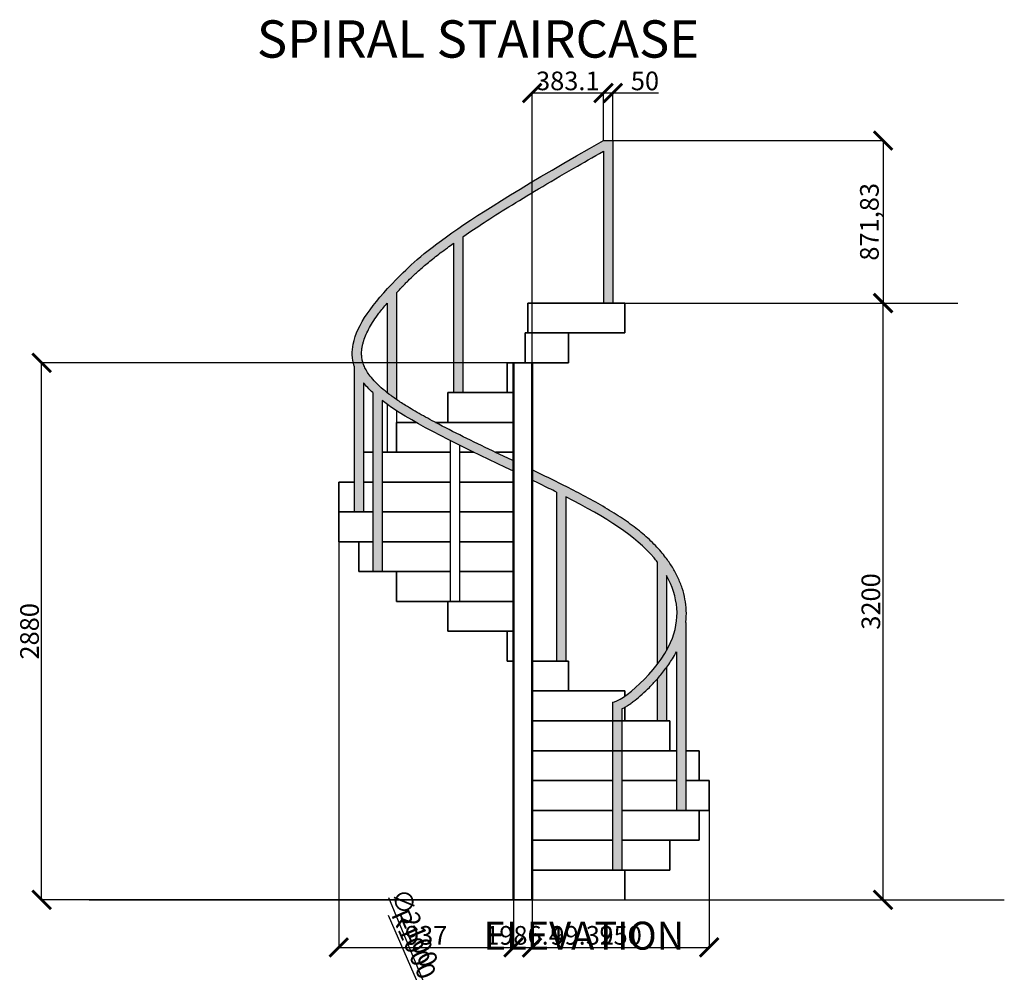
# Model space of a CAD drawing. Units: millimetres. Extents: x 210 to 5648, y 83 to 7906.
# Tile 2 of 2: x 210 to 5490, y 2798 to 7906. Entities that reach past the tile are written whole.
import ezdxf

# ---------------------------------------------------------------- set-up
doc = ezdxf.new("R2010")
doc.units = ezdxf.units.MM
for name, color, linetype, lineweight in [('A-ANNO-DIMS', 2, 'Continuous', 18), ('A-ANNO-TEXT', 240, 'Continuous', 18), ('A-COLS', 1, 'Continuous', 50), ('A-FLOR-HRAL', 4, 'Continuous', 25), ('A-FLOR-LEVL', 8, 'Continuous', 25), ('A-FLOR-PATT', 252, 'Continuous', 13), ('A-FLOR-STRS', 7, 'Continuous', 35)]:
    doc.layers.add(name, color=color, linetype=linetype, lineweight=lineweight)
doc.styles.get("Standard").update_dxf_attribs({"font": 'arial.ttf'})
doc.dimstyles.new('ISO-25', dxfattribs={"dimtxt": 100, "dimasz": 100, "dimexe": 1.25, "dimexo": 0.625, "dimtad": 1, "dimtxsty": 'Standard', "dimblk": 'ARCHTICK', "dimcen": 2.5, "dimclrd": 2, "dimclre": 5, "dimclrt": 1, "dimadec": 0, "dimazin": 0, "dimtfac": 1, "dimtmove": 0, "dimatfit": 3, "dimfxl": 1, "dimarcsym": 0})

# ---------------------------------------------------------------- blocks, each defined once
blk = doc.blocks.new('_ArchTick')
at = {"color": 0, "linetype": 'ByBlock', "const_width": 0.15}
blk.add_lwpolyline([(-0.5, -0.5), (0.5, 0.5)], dxfattribs=at)
blk = doc.blocks.new('*D4')
at = {"layer": 'A-ANNO-DIMS', "color": 0, "lineweight": -2, "transparency": 16777216}
for p, q in [((4348, 6386.1), (4839.8, 6386.1)), ((4838.6, 6386.1), (4838.6, 3186.1)), ((4348, 3186.1), (4839.8, 3186.1))]:
    blk.add_line(p, q, dxfattribs=at)
at = {"layer": 'Defpoints', "color": 0, "transparency": 16777216}
for p in [(4347.4, 6386.1), (4347.4, 3186.1), (4838.6, 3186.1)]:
    blk.add_point(p, dxfattribs=at)
at = {"layer": 'A-ANNO-DIMS', "color": 0, "lineweight": -2, "transparency": 16777216, "xscale": 100, "yscale": 100, "zscale": 100}
for p, rotation in [((4838.6, 6386.1), 90), ((4838.6, 3186.1), 270)]:
    blk.add_blockref('_ArchTick', p, dxfattribs=dict(at, rotation=rotation))
at = {"layer": 'A-ANNO-DIMS', "color": 0, "transparency": 16777216, "insert": (4786.9, 4786.1), "char_height": 100, "attachment_point": 5, "rotation": 90}
blk.add_mtext('3200', dxfattribs=at)
blk = doc.blocks.new('*D5')
at = {"layer": 'A-ANNO-DIMS', "color": 0, "lineweight": -2, "transparency": 16777216}
for p, q in [((3391.1, 7257.9), (4841.1, 7257.9)), ((4839.8, 7257.9), (4839.8, 6386.1)), ((3391.1, 6386.1), (4841.1, 6386.1))]:
    blk.add_line(p, q, dxfattribs=at)
at = {"layer": 'Defpoints', "color": 0, "transparency": 16777216}
for p in [(3390.5, 7257.9), (3390.5, 6386.1), (4839.8, 6386.1)]:
    blk.add_point(p, dxfattribs=at)
at = {"layer": 'A-ANNO-DIMS', "color": 0, "lineweight": -2, "transparency": 16777216, "xscale": 100, "yscale": 100, "zscale": 100}
for p, rotation in [((4839.8, 7257.9), 90), ((4839.8, 6386.1), 270)]:
    blk.add_blockref('_ArchTick', p, dxfattribs=dict(at, rotation=rotation))
at = {"layer": 'A-ANNO-DIMS', "color": 0, "transparency": 16777216, "insert": (4779.1, 6822), "char_height": 100, "attachment_point": 5, "rotation": 90}
blk.add_mtext('871,83', dxfattribs=at)
blk = doc.blocks.new('*D9')
at = {"layer": 'A-ANNO-DIMS', "color": 5, "lineweight": -2, "transparency": 16777216}
for p, q in [((2957.4, 6066.7), (2957.4, 7514.2)), ((3340.5, 7258.6), (3340.5, 7514.2))]:
    blk.add_line(p, q, dxfattribs=at)
at = {"layer": 'A-ANNO-DIMS', "color": 2, "lineweight": -2, "transparency": 16777216}
blk.add_line((2957.4, 7512.9), (3340.5, 7512.9), dxfattribs=at)
at = {"layer": 'Defpoints', "color": 0, "transparency": 16777216}
for p in [(3340.5, 7512.9), (3340.5, 7257.9), (2957.4, 6066.1)]:
    blk.add_point(p, dxfattribs=at)
at = {"layer": 'A-ANNO-DIMS', "color": 2, "lineweight": -2, "transparency": 16777216, "xscale": 100, "yscale": 100, "zscale": 100, "rotation": 180}
blk.add_blockref('_ArchTick', (2957.4, 7512.9), dxfattribs=at)
at = {"layer": 'A-ANNO-DIMS', "color": 2, "lineweight": -2, "transparency": 16777216, "xscale": 100, "yscale": 100, "zscale": 100}
blk.add_blockref('_ArchTick', (3340.5, 7512.9), dxfattribs=at)
at = {"layer": 'A-ANNO-DIMS', "color": 1, "transparency": 16777216, "insert": (3149, 7564.7), "char_height": 100, "attachment_point": 5}
blk.add_mtext('383.1', dxfattribs=at)
blk = doc.blocks.new('*D10')
at = {"layer": 'A-ANNO-DIMS', "color": 5, "lineweight": -2, "transparency": 16777216}
for p, q in [((3340.5, 7258.6), (3340.5, 7514.2)), ((3390.5, 7258.6), (3390.5, 7514.2))]:
    blk.add_line(p, q, dxfattribs=at)
at = {"layer": 'A-ANNO-DIMS', "color": 2, "lineweight": -2, "transparency": 16777216}
for p, q in [((3340.5, 7512.9), (3390.5, 7512.9)), ((3390.5, 7512.9), (3634.7, 7512.9))]:
    blk.add_line(p, q, dxfattribs=at)
at = {"layer": 'Defpoints', "color": 0, "transparency": 16777216}
for p in [(3390.5, 7512.9), (3340.5, 7257.9), (3390.5, 7257.9)]:
    blk.add_point(p, dxfattribs=at)
at = {"layer": 'A-ANNO-DIMS', "color": 2, "lineweight": -2, "transparency": 16777216, "xscale": 100, "yscale": 100, "zscale": 100, "rotation": 180}
blk.add_blockref('_ArchTick', (3340.5, 7512.9), dxfattribs=at)
at = {"layer": 'A-ANNO-DIMS', "color": 2, "lineweight": -2, "transparency": 16777216, "xscale": 100, "yscale": 100, "zscale": 100}
blk.add_blockref('_ArchTick', (3390.5, 7512.9), dxfattribs=at)
at = {"layer": 'A-ANNO-DIMS', "color": 1, "transparency": 16777216, "insert": (3562.6, 7564.6), "char_height": 100, "attachment_point": 5}
blk.add_mtext('50', dxfattribs=at)
blk = doc.blocks.new('*D11')
at = {"layer": 'A-ANNO-DIMS', "color": 5, "lineweight": -2, "transparency": 16777216}
for p, q in [((2957.4, 3825.5), (2957.4, 2929.9)), ((3907.4, 3825.5), (3907.4, 2929.9))]:
    blk.add_line(p, q, dxfattribs=at)
at = {"layer": 'A-ANNO-DIMS', "color": 2, "lineweight": -2, "transparency": 16777216}
blk.add_line((2957.4, 2931.1), (3907.4, 2931.1), dxfattribs=at)
at = {"layer": 'Defpoints', "color": 0, "transparency": 16777216}
for p in [(2957.4, 3826.1), (3907.4, 3826.1), (3907.4, 2931.1)]:
    blk.add_point(p, dxfattribs=at)
at = {"layer": 'A-ANNO-DIMS', "color": 2, "lineweight": -2, "transparency": 16777216, "xscale": 100, "yscale": 100, "zscale": 100, "rotation": 180}
blk.add_blockref('_ArchTick', (2957.4, 2931.1), dxfattribs=at)
at = {"layer": 'A-ANNO-DIMS', "color": 2, "lineweight": -2, "transparency": 16777216, "xscale": 100, "yscale": 100, "zscale": 100}
blk.add_blockref('_ArchTick', (3907.4, 2931.1), dxfattribs=at)
at = {"layer": 'A-ANNO-DIMS', "color": 1, "transparency": 16777216, "insert": (3432.4, 2982.8), "char_height": 100, "attachment_point": 5}
blk.add_mtext('950', dxfattribs=at)
blk = doc.blocks.new('*D12')
at = {"layer": 'A-ANNO-DIMS', "color": 5, "lineweight": -2, "transparency": 16777216}
for p, q in [((1921, 5105.5), (1921, 2929.9)), ((2858.1, 5105.5), (2858.1, 2929.9))]:
    blk.add_line(p, q, dxfattribs=at)
at = {"layer": 'A-ANNO-DIMS', "color": 2, "lineweight": -2, "transparency": 16777216}
blk.add_line((1921, 2931.1), (2858.1, 2931.1), dxfattribs=at)
at = {"layer": 'Defpoints', "color": 0, "transparency": 16777216}
for p in [(1921, 5106.1), (2858.1, 5106.1), (2858.1, 2931.1)]:
    blk.add_point(p, dxfattribs=at)
at = {"layer": 'A-ANNO-DIMS', "color": 2, "lineweight": -2, "transparency": 16777216, "xscale": 100, "yscale": 100, "zscale": 100, "rotation": 180}
blk.add_blockref('_ArchTick', (1921, 2931.1), dxfattribs=at)
at = {"layer": 'A-ANNO-DIMS', "color": 2, "lineweight": -2, "transparency": 16777216, "xscale": 100, "yscale": 100, "zscale": 100}
blk.add_blockref('_ArchTick', (2858.1, 2931.1), dxfattribs=at)
at = {"layer": 'A-ANNO-DIMS', "color": 1, "transparency": 16777216, "insert": (2389.6, 2982.8), "char_height": 100, "attachment_point": 5}
blk.add_mtext('937', dxfattribs=at)
blk = doc.blocks.new('*D13')
at = {"layer": 'A-ANNO-DIMS', "color": 5, "lineweight": -2, "transparency": 16777216}
for p, q in [((2858.1, 3185.5), (2858.1, 2929.9)), ((2957.4, 3185.5), (2957.4, 2929.9))]:
    blk.add_line(p, q, dxfattribs=at)
at = {"layer": 'A-ANNO-DIMS', "color": 2, "lineweight": -2, "transparency": 16777216}
for p, q in [((2858.1, 2931.1), (2957.4, 2931.1)), ((2957.4, 2931.1), (3395.1, 2931.1))]:
    blk.add_line(p, q, dxfattribs=at)
at = {"layer": 'Defpoints', "color": 0, "transparency": 16777216}
for p in [(2858.1, 3186.1), (2957.4, 3186.1), (2957.4, 2931.1)]:
    blk.add_point(p, dxfattribs=at)
at = {"layer": 'A-ANNO-DIMS', "color": 2, "lineweight": -2, "transparency": 16777216, "xscale": 100, "yscale": 100, "zscale": 100, "rotation": 180}
blk.add_blockref('_ArchTick', (2858.1, 2931.1), dxfattribs=at)
at = {"layer": 'A-ANNO-DIMS', "color": 2, "lineweight": -2, "transparency": 16777216, "xscale": 100, "yscale": 100, "zscale": 100}
blk.add_blockref('_ArchTick', (2957.4, 2931.1), dxfattribs=at)
at = {"layer": 'A-ANNO-DIMS', "color": 1, "transparency": 16777216, "insert": (3226.2, 2982.8), "char_height": 100, "attachment_point": 5}
blk.add_mtext('99.32', dxfattribs=at)
blk = doc.blocks.new('*D14')
at = {"layer": 'A-ANNO-DIMS', "color": 5, "lineweight": -2, "transparency": 16777216}
for p, q in [((1921, 5265.5), (1921, 2929.9)), ((3907.4, 3665.5), (3907.4, 2929.9))]:
    blk.add_line(p, q, dxfattribs=at)
at = {"layer": 'A-ANNO-DIMS', "color": 2, "lineweight": -2, "transparency": 16777216}
blk.add_line((1921, 2931.1), (3907.4, 2931.1), dxfattribs=at)
at = {"layer": 'Defpoints', "color": 0, "transparency": 16777216}
for p in [(1921, 5266.1), (3907.4, 3666.1), (3907.4, 2931.1)]:
    blk.add_point(p, dxfattribs=at)
at = {"layer": 'A-ANNO-DIMS', "color": 2, "lineweight": -2, "transparency": 16777216, "xscale": 100, "yscale": 100, "zscale": 100, "rotation": 180}
blk.add_blockref('_ArchTick', (1921, 2931.1), dxfattribs=at)
at = {"layer": 'A-ANNO-DIMS', "color": 2, "lineweight": -2, "transparency": 16777216, "xscale": 100, "yscale": 100, "zscale": 100}
blk.add_blockref('_ArchTick', (3907.4, 2931.1), dxfattribs=at)
at = {"layer": 'A-ANNO-DIMS', "color": 1, "transparency": 16777216, "insert": (2914.2, 2982.8), "char_height": 100, "attachment_point": 5}
blk.add_mtext('1986.4', dxfattribs=at)
blk = doc.blocks.new('*D15')
at = {"layer": 'A-ANNO-DIMS', "color": 5, "lineweight": -2, "transparency": 16777216}
for p, q in [((2956.8, 6066.1), (326.4, 6066.1)), ((2956.8, 3186.1), (326.4, 3186.1))]:
    blk.add_line(p, q, dxfattribs=at)
at = {"layer": 'A-ANNO-DIMS', "color": 2, "lineweight": -2, "transparency": 16777216}
blk.add_line((327.6, 3186.1), (327.6, 6066.1), dxfattribs=at)
at = {"layer": 'Defpoints', "color": 0, "transparency": 16777216}
for p in [(327.6, 6066.1), (2957.4, 6066.1), (2957.4, 3186.1)]:
    blk.add_point(p, dxfattribs=at)
at = {"layer": 'A-ANNO-DIMS', "color": 2, "lineweight": -2, "transparency": 16777216, "xscale": 100, "yscale": 100, "zscale": 100}
for p, rotation in [((327.6, 6066.1), 90), ((327.6, 3186.1), 270)]:
    blk.add_blockref('_ArchTick', p, dxfattribs=dict(at, rotation=rotation))
at = {"layer": 'A-ANNO-DIMS', "color": 1, "transparency": 16777216, "insert": (275.9, 4626.1), "char_height": 100, "attachment_point": 5, "rotation": 90}
blk.add_mtext('2880', dxfattribs=at)
blk = doc.blocks.new('*D16')
at = {"layer": 'A-ANNO-DIMS', "color": 2, "lineweight": -2, "transparency": 16777216}
for p in [(2187.7, 3199), (3308.5, 487.3)]:
    blk.add_line(p, (2506.3, 2428.1), dxfattribs=at)
at = {"layer": 'Defpoints', "color": 0, "transparency": 16777216}
for p in [(2506.3, 2428.1), (3308.5, 487.3)]:
    blk.add_point(p, dxfattribs=at)
at = {"layer": 'A-ANNO-DIMS', "color": 2, "lineweight": -2, "transparency": 16777216, "xscale": 100, "yscale": 100, "zscale": 100}
for p, rotation in [((2506.3, 2428.1), 292.4567190753457), ((3308.5, 487.3), 112.4567190753456)]:
    blk.add_blockref('_ArchTick', p, dxfattribs=dict(at, rotation=rotation))
at = {"layer": 'A-ANNO-DIMS', "color": 1, "transparency": 16777216, "insert": (2316, 3031.1), "char_height": 100, "attachment_point": 5, "rotation": 292.4567}
blk.add_mtext('∅2100', dxfattribs=at)
blk = doc.blocks.new('*D17')
at = {"layer": 'A-ANNO-DIMS', "color": 2, "lineweight": -2, "transparency": 16777216}
for p in [(2185.3, 3103.9), (2907.4, 1457.7)]:
    blk.add_line(p, (2505.7, 2373.5), dxfattribs=at)
at = {"layer": 'Defpoints', "color": 0, "transparency": 16777216}
for p in [(2505.7, 2373.5), (2907.4, 1457.7)]:
    blk.add_point(p, dxfattribs=at)
at = {"layer": 'A-ANNO-DIMS', "color": 2, "lineweight": -2, "transparency": 16777216, "xscale": 100, "yscale": 100, "zscale": 100, "rotation": 293.6842151788714}
blk.add_blockref('_ArchTick', (2505.7, 2373.5), dxfattribs=at)
at = {"layer": 'A-ANNO-DIMS', "color": 1, "transparency": 16777216, "insert": (2312, 2943.7), "char_height": 100, "attachment_point": 5, "rotation": 293.6842}
blk.add_mtext('R1000', dxfattribs=at)

msp = doc.modelspace()

# ---------------------------------------------------------------- hatches: boundary and pattern name
at = {"layer": 'A-FLOR-PATT'}
h = msp.add_hatch(color=256, dxfattribs=at)
h.dxf.hatch_style = 1
edge = h.paths.add_edge_path()
edge.add_spline(control_points=[(2230.323, 6441.345), (2237.214, 6448.743), (2244.288, 6456.237), (2254.94, 6467.39), (2258.378, 6470.97), (2264.36, 6477.168), (2266.887, 6479.777), (2271.968, 6485.002), (2274.525, 6487.621), (2282.261, 6495.505), (2287.506, 6500.797), (2303.631, 6516.855), (2314.902, 6527.799), (2341.337, 6552.563), (2356.838, 6566.548), (2391.369, 6596.276), (2410.399, 6612.017), (2453.073, 6645.774), (2476.716, 6663.789), (2513.779, 6690.939), (2524.82, 6698.916), (2536.348, 6707.128)], knot_values=[5.90489117, 5.90489117, 5.90489117, 5.90489117, 5.96373465, 5.96373465, 5.9913029, 5.9913029, 6.0111685, 6.0111685, 6.03103409, 6.03103409, 6.07076529, 6.07076529, 6.15022769, 6.15022769, 6.24382005, 6.24382005, 6.33741241, 6.33741241, 6.43100477, 6.43100477, 6.46843693, 6.46843693, 6.46843693, 6.46843693], degree=3, periodic=0)
edge.add_line((2536.348, 6707.128), (2536.348, 5906.102))
edge.add_line((2536.348, 5906.102), (2586.348, 5906.102))
edge.add_line((2586.348, 5906.102), (2586.348, 6742.111))
edge.add_spline(control_points=[(2586.348, 6742.111), (2588.096, 6743.314), (2589.855, 6744.521), (2657.298, 6790.759), (2736.51, 6842.312), (2930.306, 6962.284), (3044.888, 7030.703), (3231.366, 7138.39), (3284.371, 7168.696), (3340.522, 7200.493)], knot_values=[6.51952859, 6.51952859, 6.51952859, 6.51952859, 6.52459713, 6.52459713, 6.71284254, 6.71284254, 6.90108795, 6.90108795, 6.97017576, 6.97017576, 6.97017576, 6.97017576], degree=3, periodic=0)
edge.add_line((3340.522, 7200.493), (3340.522, 6386.102))
edge.add_line((3340.522, 6386.102), (3390.522, 6386.102))
edge.add_line((3390.522, 6386.102), (3390.522, 7257.935))
edge.add_line((3390.522, 7257.935), (3340.522, 7257.935))
edge.add_spline(control_points=[(3340.522, 7257.935), (2981.042, 7054.904), (2746.784, 6911.149), (2586.348, 6802.632)], knot_values=[6.54582273, 6.54582273, 6.54582273, 6.54582273, 6.98017889, 6.98017889, 6.98017889, 6.98017889], degree=3, periodic=0)
edge.add_spline(control_points=[(2586.348, 6802.632), (2384.739, 6666.266), (2143.904, 6437.657), (1990.881, 6234.097), (1991.101, 6088.759), (2003.82, 6048.816)], knot_values=[4.63745133, 4.63745133, 4.63745133, 4.63745133, 5.18327406, 6.18327406, 6.54582273, 6.54582273, 6.54582273, 6.54582273], degree=3, periodic=0)
edge.add_line((2003.82, 6048.816), (2003.82, 5266.102))
edge.add_line((2003.82, 5266.102), (2053.82, 5266.102))
edge.add_line((2053.82, 5266.102), (2053.82, 5958.825))
edge.add_spline(control_points=[(2053.82, 5958.825), (2067.467, 5941.686), (2083.758, 5924.189), (2103.017, 5906.251)], knot_values=[4.2265259, 4.2265259, 4.2265259, 4.2265259, 4.37281832, 4.37281832, 4.37281832, 4.37281832], degree=3, periodic=0)
edge.add_line((2103.017, 5906.251), (2103.017, 4946.102))
edge.add_line((2103.017, 4946.102), (2153.017, 4946.102))
edge.add_line((2153.017, 4946.102), (2153.017, 5863.924))
edge.add_spline(control_points=[(2153.017, 5863.924), (2161.695, 5857.182), (2170.791, 5850.374), (2180.323, 5843.497)], knot_values=[4.06087851, 4.06087851, 4.06087851, 4.06087851, 4.11370793, 4.11370793, 4.11370793, 4.11370793], degree=3, periodic=0)
edge.add_spline(control_points=[(2180.323, 5843.497), (2191.306, 5835.571), (2207.618, 5824.257), (2225.126, 5812.747), (2230.323, 5809.378)], knot_values=[3.97497946, 3.97497946, 3.97497946, 3.97497946, 4.03585797, 4.06087851, 4.06087851, 4.06087851, 4.06087851], degree=3, periodic=0)
edge.add_spline(control_points=[(2230.323, 5809.378), (2262.049, 5788.814), (2297.407, 5767.659), (2335.496, 5746.102)], knot_values=[3.8222376, 3.8222376, 3.8222376, 3.8222376, 3.97497946, 3.97497946, 3.97497946, 3.97497946], degree=3, periodic=0)
edge.add_spline(control_points=[(2335.496, 5746.102), (2391.715, 5714.285), (2453.883, 5681.595), (2519.103, 5648.642)], knot_values=[3.59679122, 3.59679122, 3.59679122, 3.59679122, 3.8222376, 3.8222376, 3.8222376, 3.8222376], degree=3, periodic=0)
edge.add_spline(control_points=[(2519.103, 5648.642), (2535.59, 5640.312), (2552.272, 5631.965), (2569.103, 5623.611)], knot_values=[3.53979942, 3.53979942, 3.53979942, 3.53979942, 3.59679122, 3.59679122, 3.59679122, 3.59679122], degree=3, periodic=0)
edge.add_spline(control_points=[(2569.103, 5623.611), (2594.283, 5611.112), (2619.795, 5598.598), (2645.481, 5586.102)], knot_values=[3.45453406, 3.45453406, 3.45453406, 3.45453406, 3.53979942, 3.53979942, 3.53979942, 3.53979942], degree=3, periodic=0)
edge.add_spline(control_points=[(2645.481, 5586.102), (2716.113, 5551.741), (2788.067, 5517.513), (2858.085, 5484.105)], knot_values=[3.22007561, 3.22007561, 3.22007561, 3.22007561, 3.45453406, 3.45453406, 3.45453406, 3.45453406], degree=3, periodic=0)
edge.add_line((2858.085, 5484.105), (2858.085, 5539.503))
edge.add_spline(control_points=[(2858.085, 5539.503), (2827.328, 5554.173), (2796.294, 5568.971), (2763.683, 5584.596), (2762.111, 5585.349), (2760.54, 5586.102)], knot_values=[3.24403738, 3.24403738, 3.24403738, 3.24403738, 3.34649082, 3.34649082, 3.35167775, 3.35167775, 3.35167775, 3.35167775], degree=3, periodic=0)
edge.add_spline(control_points=[(2760.54, 5586.102), (2709.179, 5610.722), (2657.838, 5635.532), (2556.156, 5685.75), (2505.893, 5711.154), (2452.051, 5739.479), (2445.783, 5742.795), (2439.567, 5746.102)], knot_values=[3.35167775, 3.35167775, 3.35167775, 3.35167775, 3.52120514, 3.52120514, 3.69591945, 3.69591945, 3.71913913, 3.71913913, 3.71913913, 3.71913913], degree=3, periodic=0)
edge.add_spline(control_points=[(2439.567, 5746.102), (2413.223, 5760.121), (2387.808, 5773.996), (2333.635, 5804.555), (2305.503, 5821.132), (2269.838, 5843.389), (2260.321, 5849.471), (2243.996, 5860.182), (2237.049, 5864.841), (2230.323, 5869.455)], knot_values=[3.71913913, 3.71913913, 3.71913913, 3.71913913, 3.81754541, 3.81754541, 3.93917136, 3.93917136, 3.98562211, 3.98562211, 4.02206941, 4.02206941, 4.02206941, 4.02206941], degree=3, periodic=0)
edge.add_spline(control_points=[(2230.323, 5869.455), (2228.581, 5870.65), (2226.854, 5871.842), (2216.818, 5878.81), (2208.841, 5884.519), (2193.939, 5895.516), (2186.982, 5900.811), (2180.323, 5906.041)], knot_values=[4.02206941, 4.02206941, 4.02206941, 4.02206941, 4.03150589, 4.03150589, 4.07738967, 4.07738967, 4.12101551, 4.12101551, 4.12101551, 4.12101551], degree=3, periodic=0)
edge.add_spline(control_points=[(2180.323, 5906.041), (2172.974, 5911.812), (2165.987, 5917.504), (2144.201, 5935.928), (2130.878, 5948.324), (2107.575, 5972.254), (2097.596, 5983.788), (2082.165, 6003.935), (2076.218, 6012.694), (2066.046, 6029.662), (2061.82, 6037.87), (2054.825, 6053.836), (2052.053, 6061.594), (2047.722, 6076.837), (2046.161, 6084.324), (2044.077, 6099.249), (2043.555, 6106.689), (2043.453, 6121.725), (2043.876, 6129.321), (2045.161, 6140.725), (2045.674, 6144.419), (2046.77, 6151.11), (2047.318, 6154.096), (2048.532, 6160.108), (2049.197, 6163.123), (2051.367, 6172.201), (2053.047, 6178.299), (2058.458, 6195.653), (2062.743, 6207.05), (2072.966, 6230.362), (2078.906, 6242.275), (2092.479, 6266.689), (2100.113, 6279.188), (2117.083, 6304.82), (2126.418, 6317.953), (2149.772, 6348.873), (2164.362, 6366.889), (2180.323, 6385.536)], knot_values=[4.12101551, 4.12101551, 4.12101551, 4.12101551, 4.16915722, 4.16915722, 4.27905295, 4.27905295, 4.38894868, 4.38894868, 4.4785858, 4.4785858, 4.56822292, 4.56822292, 4.65786004, 4.65786004, 4.74749715, 4.74749715, 4.83713427, 4.83713427, 4.92677139, 4.92677139, 4.96916501, 4.96916501, 5.00281636, 5.00281636, 5.03646771, 5.03646771, 5.1037704, 5.1037704, 5.22617685, 5.22617685, 5.34858331, 5.34858331, 5.47098976, 5.47098976, 5.59339622, 5.59339622, 5.75191312, 5.75191312, 5.75191312, 5.75191312], degree=3, periodic=0)
edge.add_line((2180.323, 6385.536), (2180.323, 5906.041))
edge.add_spline(control_points=[(2180.323, 5906.041), (2186.982, 5900.811), (2193.939, 5895.516), (2208.841, 5884.519), (2216.818, 5878.81), (2226.854, 5871.842), (2228.581, 5870.65), (2230.323, 5869.455)], knot_values=[4.02206941, 4.02206941, 4.02206941, 4.02206941, 4.06569525, 4.06569525, 4.11157903, 4.11157903, 4.12101551, 4.12101551, 4.12101551, 4.12101551], degree=3, periodic=0)
edge.add_line((2230.323, 5869.455), (2230.323, 6441.345))
h = msp.add_hatch(color=256, dxfattribs=at)
h.dxf.hatch_style = 1
edge = h.paths.add_edge_path()
edge.add_spline(control_points=[(3781.861, 4673.689), (3781.945, 4674.405), (3782.026, 4675.121), (3784.412, 4696.601), (3785.116, 4717.29), (3783.499, 4758.294), (3781.181, 4778.609), (3773.753, 4818.679), (3768.645, 4838.436), (3755.889, 4877.258), (3748.241, 4896.325), (3730.647, 4933.684), (3720.701, 4951.976), (3698.73, 4987.728), (3686.706, 5005.188), (3665.888, 5032.519), (3657.69, 5042.669), (3629.972, 5075.136), (3609.122, 5096.786), (3564.067, 5138.823), (3539.863, 5159.212), (3487.997, 5199.2), (3460.335, 5218.801), (3401.383, 5257.702), (3370.093, 5277.003), (3303.681, 5315.786), (3268.56, 5335.267), (3214.918, 5363.864), (3198.024, 5372.72), (3146.116, 5399.538), (3109.873, 5417.749), (3035.144, 5454.562), (2996.77, 5473.13), (2957.403, 5492.028)], knot_values=[1.23691972, 1.23691972, 1.23691972, 1.23691972, 1.24089242, 1.24089242, 1.35609231, 1.35609231, 1.4712922, 1.4712922, 1.58649209, 1.58649209, 1.70169198, 1.70169198, 1.81689187, 1.81689187, 1.93209176, 1.93209176, 2.00188444, 2.00188444, 2.15904986, 2.15904986, 2.31621528, 2.31621528, 2.47338069, 2.47338069, 2.63054611, 2.63054611, 2.78771153, 2.78771153, 2.85749508, 2.85749508, 2.99706219, 2.99706219, 3.13226931, 3.13226931, 3.13226931, 3.13226931], degree=3, periodic=0)
edge.add_line((2957.403, 5492.028), (2957.403, 5436.549))
edge.add_spline(control_points=[(2957.403, 5436.549), (2988.252, 5421.693), (3032.736, 5400.104), (3074.935, 5379.185), (3088.331, 5372.491)], knot_values=[2.94879845, 2.94879845, 2.94879845, 2.94879845, 3.05611076, 3.10731232, 3.10731232, 3.10731232, 3.10731232], degree=3, periodic=0)
edge.add_line((3088.331, 5372.491), (3088.331, 4466.102))
edge.add_line((3088.331, 4466.102), (3138.331, 4466.102))
edge.add_line((3138.331, 4466.102), (3138.331, 5347.228))
edge.add_spline(control_points=[(3138.331, 5347.228), (3359.291, 5234.253), (3520.089, 5131.778), (3622.943, 5006.062), (3628.268, 4999.279)], knot_values=[1.95009854, 1.95009854, 1.95009854, 1.95009854, 2.83374836, 2.88364982, 2.88364982, 2.88364982, 2.88364982], degree=3, periodic=0)
edge.add_line((3628.268, 4999.279), (3628.268, 4448.446))
edge.add_spline(control_points=[(3628.268, 4448.446), (3646.667, 4472.431), (3663.687, 4497.441), (3678.268, 4522.82)], knot_values=[0.74965342, 0.74965342, 0.74965342, 0.74965342, 0.90958311, 0.90958311, 0.90958311, 0.90958311], degree=3, periodic=0)
edge.add_line((3678.268, 4522.82), (3678.268, 4924.666))
edge.add_spline(control_points=[(3678.268, 4924.666), (3740.506, 4813.344), (3757.759, 4675.257), (3686.512, 4537.169), (3678.268, 4522.82)], knot_values=[0.90958311, 0.90958311, 0.90958311, 0.90958311, 1.68221449, 1.77263138, 1.77263138, 1.77263138, 1.77263138], degree=3, periodic=0)
edge.add_spline(control_points=[(3678.268, 4522.82), (3663.687, 4497.441), (3646.667, 4472.431), (3628.268, 4448.446)], knot_values=[0.74965342, 0.74965342, 0.74965342, 0.74965342, 0.90958311, 0.90958311, 0.90958311, 0.90958311], degree=3, periodic=0)
edge.add_spline(control_points=[(3628.268, 4448.446), (3573.149, 4376.59), (3505.665, 4313.928), (3454.351, 4278.062)], knot_values=[0.27051991, 0.27051991, 0.27051991, 0.27051991, 0.74965342, 0.74965342, 0.74965342, 0.74965342], degree=3, periodic=0)
edge.add_spline(control_points=[(3454.351, 4278.062), (3425.379, 4257.811), (3401.562, 4246.102), (3388.036, 4246.102)], knot_values=[0, 0, 0, 0, 0.27051991, 0.27051991, 0.27051991, 0.27051991], degree=3, periodic=0)
edge.add_line((3388.036, 4245.424), (3388.036, 4146.102))
edge.add_line((3388.036, 4146.102), (3438.036, 4146.102))
edge.add_line((3438.036, 4146.102), (3438.036, 4209.897))
edge.add_spline(control_points=[(3438.036, 4209.897), (3440.677, 4211.191), (3443.321, 4212.552), (3448.752, 4215.468), (3451.54, 4217.029), (3454.351, 4218.661)], knot_values=[0.13781612, 0.13781612, 0.13781612, 0.13781612, 0.1620919, 0.1620919, 0.18736587, 0.18736587, 0.18736587, 0.18736587], degree=3, periodic=0)
edge.add_spline(control_points=[(3454.351, 4218.661), (3454.757, 4218.897), (3455.163, 4219.134), (3461.214, 4222.683), (3466.96, 4226.282), (3478.698, 4234.043), (3484.688, 4238.205), (3496.903, 4247.07), (3503.128, 4251.773), (3521.788, 4266.405), (3534.509, 4277.057), (3560.369, 4300.091), (3573.506, 4312.474), (3599.764, 4338.724), (3612.886, 4352.59), (3626.606, 4368.011), (3627.438, 4368.949), (3628.268, 4369.891)], knot_values=[0.18736587, 0.18736587, 0.18736587, 0.18736587, 0.19101455, 0.19101455, 0.24163062, 0.24163062, 0.29224669, 0.29224669, 0.34286276, 0.34286276, 0.44154301, 0.44154301, 0.54022326, 0.54022326, 0.63890352, 0.63890352, 0.64528101, 0.64528101, 0.64528101, 0.64528101], degree=3, periodic=0)
edge.add_spline(control_points=[(3628.268, 4369.891), (3642.58, 4386.105), (3656.582, 4403.075), (3672.751, 4424.326), (3675.525, 4428.035), (3678.268, 4431.769)], knot_values=[0.64528101, 0.64528101, 0.64528101, 0.64528101, 0.75514118, 0.75514118, 0.77817085, 0.77817085, 0.77817085, 0.77817085], degree=3, periodic=0)
edge.add_spline(control_points=[(3678.268, 4431.769), (3689.371, 4446.881), (3699.966, 4462.403), (3717.67, 4490.805), (3725.045, 4503.562), (3731.861, 4516.498)], knot_values=[0.77817085, 0.77817085, 0.77817085, 0.77817085, 0.87137885, 0.87137885, 0.9451649, 0.9451649, 0.9451649, 0.9451649], degree=3, periodic=0)
edge.add_line((3731.861, 4516.498), (3731.861, 3666.102))
edge.add_line((3731.861, 3666.102), (3781.861, 3666.102))
edge.add_line((3781.861, 3666.102), (3781.861, 4673.689))
h.paths.add_polyline_path([(3438.036, 3986.102), (3388.036, 3986.102), (3388.036, 3346.102), (3438.036, 3346.102)])
h = msp.add_hatch(color=256, dxfattribs=at)
h.dxf.hatch_style = 1
edge = h.paths.add_edge_path()
edge.add_spline(control_points=[(3678.268, 4431.769), (3675.525, 4428.035), (3672.751, 4424.326), (3656.582, 4403.075), (3642.58, 4386.105), (3628.268, 4369.891)], knot_values=[0.64528101, 0.64528101, 0.64528101, 0.64528101, 0.66831067, 0.66831067, 0.77817085, 0.77817085, 0.77817085, 0.77817085], degree=3, periodic=0)
edge.add_line((3628.268, 4369.891), (3628.268, 4146.102))
edge.add_line((3628.268, 4146.102), (3678.268, 4146.102))
edge.add_line((3678.268, 4146.102), (3678.268, 4431.769))
h = msp.add_hatch(color=256, dxfattribs=at)
h.dxf.hatch_style = 1
h.paths.add_polyline_path([(3438.036, 4146.102), (3388.036, 4146.102), (3388.036, 3986.102), (3438.036, 3986.102)])

# ---------------------------------------------------------------- linework, layer by layer
at = {"layer": 'A-COLS'}
for p, q in [((2858.085, 5484.105), (2858.085, 6066.102)), ((2957.403, 5436.549), (2957.403, 6066.102)), ((2858.085, 3186.102), (2858.085, 5484.105)), ((2957.403, 3186.102), (2957.403, 5436.549))]:
    msp.add_line(p, q, dxfattribs=at)
at = {"layer": 'A-FLOR-HRAL'}
for p, q in [((3340.522, 7257.935), (3390.522, 7257.935)), ((3390.522, 7257.935), (3390.522, 6386.102)), ((3340.522, 7200.493), (3340.522, 6386.102)), ((2586.348, 6806.102), (2586.348, 6802.632)), ((2536.348, 6707.128), (2536.348, 5906.102)), ((2586.348, 6742.111), (2586.348, 5906.102)), ((2230.323, 6441.345), (2230.323, 5869.455)), ((2180.323, 6385.536), (2180.323, 5906.041)), ((2003.82, 6048.816), (2003.82, 5266.102)), ((2053.82, 5958.825), (2053.82, 5266.102)), ((2103.017, 5906.251), (2103.017, 4946.102)), ((2153.017, 5863.924), (2153.017, 4946.102)), ((2180.323, 5843.497), (2180.323, 5586.102)), ((2230.323, 5809.378), (2230.323, 5586.102)), ((2519.103, 5648.642), (2519.103, 4786.102)), ((2569.103, 5623.611), (2569.103, 4786.102)), ((3088.331, 5372.491), (3088.331, 4466.102)), ((3138.331, 5347.228), (3138.331, 4466.102)), ((3628.268, 4999.279), (3628.268, 4448.446)), ((3678.268, 4924.666), (3678.268, 4522.82)), ((3781.861, 4673.689), (3781.861, 3666.102)), ((3731.861, 4516.498), (3731.861, 3666.102)), ((3678.268, 4431.769), (3678.268, 4146.102)), ((3628.268, 4369.891), (3628.268, 4146.102)), ((3388.036, 4246.102), (3388.036, 3346.102)), ((3438.036, 4209.897), (3438.036, 3346.102))]:
    msp.add_line(p, q, dxfattribs=at)
for points, knots in [([(2003.82, 6048.816), (1991.101, 6088.759), (1990.881, 6234.097), (2178.733, 6483.988), (2529.31, 6799.77), (3340.522, 7257.935)], [4.63745133, 4.63745133, 4.63745133, 4.63745133, 5, 6, 6.98017889, 6.98017889, 6.98017889, 6.98017889]), ([(2586.348, 6742.111), (2588.096, 6743.314), (2589.855, 6744.521), (2657.298, 6790.759), (2736.51, 6842.312), (2930.306, 6962.284), (3044.888, 7030.703), (3231.366, 7138.39), (3284.371, 7168.696), (3340.522, 7200.493)], [6.519528589, 6.519528589, 6.519528589, 6.519528589, 6.524597131, 6.524597131, 6.712842542, 6.712842542, 6.901087953, 6.901087953, 6.970175759, 6.970175759, 6.970175759, 6.970175759]), ([(2230.323, 6441.345), (2237.214, 6448.743), (2244.288, 6456.237), (2254.94, 6467.39), (2258.378, 6470.97), (2264.36, 6477.168), (2266.887, 6479.777), (2271.968, 6485.002), (2274.525, 6487.621), (2282.261, 6495.505), (2287.506, 6500.797), (2303.631, 6516.855), (2314.902, 6527.799), (2341.337, 6552.563), (2356.838, 6566.548), (2391.369, 6596.276), (2410.399, 6612.017), (2453.073, 6645.774), (2476.716, 6663.789), (2513.779, 6690.939), (2524.82, 6698.916), (2536.348, 6707.128)], [5.904891169, 5.904891169, 5.904891169, 5.904891169, 5.963734651, 5.963734651, 5.991302897, 5.991302897, 6.011168496, 6.011168496, 6.031034094, 6.031034094, 6.070765292, 6.070765292, 6.150227687, 6.150227687, 6.243820048, 6.243820048, 6.337412409, 6.337412409, 6.43100477, 6.43100477, 6.468436926, 6.468436926, 6.468436926, 6.468436926]), ([(2858.085, 5539.503), (2827.328, 5554.173), (2796.294, 5568.971), (2712.321, 5609.204), (2659.37, 5634.775), (2556.156, 5685.75), (2505.893, 5711.154), (2425.282, 5753.561), (2393.525, 5770.771), (2333.635, 5804.555), (2305.503, 5821.132), (2269.838, 5843.389), (2260.321, 5849.471), (2242.137, 5861.402), (2233.467, 5867.25), (2216.818, 5878.81), (2208.841, 5884.519), (2185.925, 5901.43), (2172.001, 5912.418), (2144.201, 5935.928), (2130.878, 5948.324), (2107.575, 5972.254), (2097.596, 5983.788), (2082.165, 6003.935), (2076.218, 6012.694), (2066.046, 6029.662), (2061.82, 6037.87), (2054.825, 6053.836), (2052.053, 6061.594), (2047.722, 6076.837), (2046.161, 6084.324), (2044.077, 6099.249), (2043.555, 6106.689), (2043.453, 6121.725), (2043.876, 6129.321), (2045.161, 6140.725), (2045.674, 6144.419), (2046.77, 6151.11), (2047.318, 6154.096), (2048.532, 6160.108), (2049.197, 6163.123), (2051.367, 6172.201), (2053.047, 6178.299), (2058.458, 6195.653), (2062.743, 6207.05), (2072.966, 6230.362), (2078.906, 6242.275), (2092.479, 6266.689), (2100.113, 6279.188), (2117.083, 6304.82), (2126.418, 6317.953), (2149.772, 6348.873), (2164.362, 6366.889), (2180.323, 6385.536)], [3.24403738, 3.24403738, 3.24403738, 3.24403738, 3.34649082, 3.34649082, 3.52120514, 3.52120514, 3.69591945, 3.69591945, 3.81754541, 3.81754541, 3.93917136, 3.93917136, 3.98562211, 3.98562211, 4.03150589, 4.03150589, 4.07738967, 4.07738967, 4.16915722, 4.16915722, 4.27905295, 4.27905295, 4.38894868, 4.38894868, 4.4785858, 4.4785858, 4.56822292, 4.56822292, 4.65786004, 4.65786004, 4.74749715, 4.74749715, 4.83713427, 4.83713427, 4.92677139, 4.92677139, 4.96916501, 4.96916501, 5.00281636, 5.00281636, 5.03646771, 5.03646771, 5.1037704, 5.1037704, 5.22617685, 5.22617685, 5.34858331, 5.34858331, 5.47098976, 5.47098976, 5.59339622, 5.59339622, 5.75191312, 5.75191312, 5.75191312, 5.75191312]), ([(2858.085, 5484.105), (2625.173, 5595.235), (2333.744, 5732.972), (2171.694, 5849.413), (2153.017, 5863.924)], [3.220075614, 3.220075614, 3.220075614, 3.220075614, 4, 4.113707935, 4.113707935, 4.113707935, 4.113707935]), ([(3781.861, 4673.689), (3781.945, 4674.405), (3782.026, 4675.121), (3784.412, 4696.601), (3785.116, 4717.29), (3783.499, 4758.294), (3781.181, 4778.609), (3773.753, 4818.679), (3768.645, 4838.436), (3755.889, 4877.258), (3748.241, 4896.325), (3730.647, 4933.684), (3720.701, 4951.976), (3698.73, 4987.728), (3686.706, 5005.188), (3665.888, 5032.519), (3657.69, 5042.669), (3629.972, 5075.136), (3609.122, 5096.786), (3564.067, 5138.823), (3539.863, 5159.212), (3487.997, 5199.2), (3460.335, 5218.801), (3401.383, 5257.702), (3370.093, 5277.003), (3303.681, 5315.786), (3268.56, 5335.267), (3214.918, 5363.864), (3198.024, 5372.72), (3146.116, 5399.538), (3109.873, 5417.749), (3035.144, 5454.562), (2996.77, 5473.13), (2957.403, 5492.028)], [1.23691972, 1.23691972, 1.23691972, 1.23691972, 1.24089242, 1.24089242, 1.35609231, 1.35609231, 1.4712922, 1.4712922, 1.58649209, 1.58649209, 1.70169198, 1.70169198, 1.81689187, 1.81689187, 1.93209176, 1.93209176, 2.00188444, 2.00188444, 2.15904986, 2.15904986, 2.31621528, 2.31621528, 2.47338069, 2.47338069, 2.63054611, 2.63054611, 2.78771153, 2.78771153, 2.85749508, 2.85749508, 2.99706219, 2.99706219, 3.13226931, 3.13226931, 3.13226931, 3.13226931]), ([(3088.331, 5372.491), (3074.935, 5379.185), (3032.736, 5400.104), (2988.252, 5421.693), (2957.403, 5436.549)], [2.948798446, 2.948798446, 2.948798446, 2.948798446, 3, 3.107312317, 3.107312317, 3.107312317, 3.107312317]), ([(3628.268, 4999.279), (3622.943, 5006.062), (3520.089, 5131.778), (3359.291, 5234.253), (3138.331, 5347.228)], [1.950098543, 1.950098543, 1.950098543, 1.950098543, 2, 2.88364982, 2.88364982, 2.88364982, 2.88364982]), ([(3388.036, 4246.102), (3438.036, 4246.102), (3775.941, 4529.723), (3740.506, 4813.344), (3678.268, 4924.666)], [0, 0, 0, 0, 1, 1.77263138, 1.77263138, 1.77263138, 1.77263138]), ([(3438.036, 4209.897), (3440.677, 4211.191), (3443.321, 4212.552), (3449.152, 4215.683), (3452.345, 4217.481), (3461.214, 4222.683), (3466.96, 4226.282), (3478.698, 4234.043), (3484.688, 4238.205), (3496.903, 4247.07), (3503.128, 4251.773), (3521.788, 4266.405), (3534.509, 4277.057), (3560.369, 4300.091), (3573.506, 4312.474), (3599.764, 4338.724), (3612.886, 4352.59), (3640.952, 4384.136), (3655.806, 4402.055), (3684.092, 4439.231), (3697.525, 4458.487), (3717.67, 4490.805), (3725.045, 4503.562), (3731.861, 4516.498)], [0.137816124, 0.137816124, 0.137816124, 0.137816124, 0.162091895, 0.162091895, 0.191014553, 0.191014553, 0.24163062, 0.24163062, 0.292246688, 0.292246688, 0.342862756, 0.342862756, 0.441543009, 0.441543009, 0.540223263, 0.540223263, 0.638903516, 0.638903516, 0.755141182, 0.755141182, 0.871378848, 0.871378848, 0.945164896, 0.945164896, 0.945164896, 0.945164896])]:
    msp.add_open_spline(points, degree=3, knots=knots, dxfattribs=at)
msp.add_open_spline([(2103.017, 5906.251), (2083.758, 5924.189), (2067.467, 5941.686), (2053.82, 5958.825)], degree=3, dxfattribs=at)
at = {"layer": 'A-FLOR-LEVL'}
for p, q in [((3454.351, 6386.102), (5240.471, 6386.102)), ((582.601, 3186.102), (5489.504, 3186.102))]:
    msp.add_line(p, q, dxfattribs=at)
at = {"layer": 'A-FLOR-STRS'}
for p, q in [((2934.75, 6386.102), (3454.351, 6386.102)), ((2934.75, 6386.102), (2934.75, 6226.102)), ((3454.351, 6386.102), (3454.351, 6226.102)), ((2919.677, 6226.102), (3454.351, 6226.102)), ((2919.677, 6226.102), (2919.677, 6066.102)), ((3152.888, 6226.102), (3152.888, 6066.102)), ((2824.823, 6066.102), (2824.823, 5906.102)), ((2824.823, 6066.102), (3152.888, 6066.102)), ((2505.707, 5906.102), (2858.085, 5906.102)), ((2505.707, 5746.102), (2505.707, 5906.102)), ((2230.121, 5746.102), (2335.496, 5746.102)), ((2230.121, 5746.102), (2230.121, 5586.102)), ((2439.567, 5746.102), (2858.085, 5746.102)), ((2053.82, 5586.102), (2103.017, 5586.102)), ((2153.017, 5586.102), (2519.103, 5586.102)), ((2569.103, 5586.102), (2645.481, 5586.102)), ((2760.54, 5586.102), (2858.085, 5586.102)), ((1921.041, 5426.102), (1921.041, 5106.102)), ((1921.041, 5426.102), (2003.82, 5426.102)), ((2053.82, 5426.102), (2103.017, 5426.102)), ((2153.017, 5426.102), (2519.103, 5426.102)), ((2569.103, 5426.102), (2858.085, 5426.102)), ((1921.041, 5266.102), (1921.041, 5106.102)), ((1921.041, 5266.102), (2103.017, 5266.102)), ((2153.017, 5266.102), (2519.103, 5266.102)), ((2569.103, 5266.102), (2858.085, 5266.102)), ((1921.041, 5106.102), (2103.017, 5106.102)), ((2027.929, 5106.102), (2027.929, 4946.102)), ((2027.929, 5106.102), (2027.929, 4946.102)), ((2153.017, 5106.102), (2519.103, 5106.102)), ((2569.103, 5106.102), (2858.085, 5106.102)), ((2027.929, 4946.102), (2519.103, 4946.102)), ((2230.121, 4946.102), (2230.121, 4786.102)), ((2569.103, 4946.102), (2858.085, 4946.102)), ((2230.121, 4786.102), (2858.085, 4786.102)), ((2505.707, 4626.102), (2505.707, 4786.102)), ((2505.707, 4626.102), (2858.085, 4626.102)), ((2824.823, 4466.102), (2824.823, 4626.102)), ((2824.823, 4466.102), (2858.085, 4466.102)), ((2957.403, 4466.102), (3152.888, 4466.102)), ((3152.888, 4466.102), (3152.888, 4306.102)), ((2957.403, 4306.102), (3454.351, 4306.102)), ((3454.351, 4306.102), (3454.351, 4278.062)), ((3454.351, 4218.661), (3454.351, 4146.102)), ((2957.403, 4146.102), (3696.543, 4146.102)), ((3696.543, 3986.102), (3696.543, 4146.102)), ((2957.403, 3986.102), (3731.861, 3986.102)), ((3781.861, 3986.102), (3853.22, 3986.102)), ((3853.22, 3986.102), (3853.22, 3826.102)), ((2957.403, 3826.102), (3388.036, 3826.102)), ((3438.036, 3826.102), (3731.861, 3826.102)), ((3781.861, 3826.102), (3907.403, 3826.102)), ((3907.403, 3826.102), (3907.403, 3666.102)), ((2957.403, 3666.102), (3388.036, 3666.102)), ((3438.036, 3666.102), (3907.403, 3666.102)), ((3853.22, 3666.102), (3853.22, 3506.102)), ((2957.403, 3506.102), (3388.036, 3506.102)), ((3438.036, 3506.102), (3853.22, 3506.102)), ((3696.543, 3506.102), (3696.543, 3346.102)), ((2957.403, 3346.102), (3696.543, 3346.102)), ((3454.351, 3346.102), (3454.351, 3186.102))]:
    msp.add_line(p, q, dxfattribs=at)

# ---------------------------------------------------------------- texts
at = {"layer": 'A-ANNO-TEXT', "attachment_point": 1}
for s, insert, char_height, width in [('{\\fArial|b1|i0|c0|p34;SPIRAL STAIRCASE}', (1481.957, 7902.359), 200, 3072.35378), ('{\\fArial|b1|i0|c0|p34;ELEVATION}', (2697.174, 3069.128), 150, 1371.70251)]:
    msp.add_mtext(s, dxfattribs=dict(at, insert=insert, char_height=char_height, width=width))

# ---------------------------------------------------------------- dimensions: what is measured, and where the dimension line sits
at = {"layer": 'A-ANNO-DIMS'}
for base, p1, p2, override, picture, middle in [((3340.522, 7512.935), (2957.403, 6066.102), (3340.522, 7257.935), {"dimdec": 1, "dimlfac": 1, "dimrnd": 0, "dimzin": 0, "dimdsep": 46, "dimlunit": 2}, '*D9', (3148.963, 7564.651)), ((3390.522, 7512.935), (3340.522, 7257.935), (3390.522, 7257.935), {"dimdec": 0, "dimlfac": 1, "dimrnd": 0, "dimzin": 0, "dimdsep": 46, "dimlunit": 2}, '*D10', (3562.6, 7564.617)), ((3907.403, 2931.102), (1921.041, 5266.102), (3907.403, 3666.102), {"dimdec": 1, "dimlfac": 1, "dimrnd": 0, "dimzin": 0, "dimdsep": 46, "dimlunit": 2}, '*D14', (2914.222, 2982.785)), ((2858.085, 2931.102), (1921.041, 5106.102), (2858.085, 5106.102), {"dimdec": 0, "dimlfac": 1, "dimrnd": 0, "dimzin": 0, "dimdsep": 46, "dimlunit": 2}, '*D12', (2389.563, 2982.819)), ((3907.403, 2931.102), (2957.403, 3826.102), (3907.403, 3826.102), {"dimdec": 0, "dimlfac": 1, "dimrnd": 0, "dimzin": 0, "dimdsep": 46, "dimlunit": 2}, '*D11', (3432.403, 2982.785)), ((2957.403, 2931.102), (2858.085, 3186.102), (2957.403, 3186.102), {"dimdec": 2, "dimlfac": 1, "dimrnd": 0, "dimzin": 0, "dimdsep": 46, "dimlunit": 2}, '*D13', (3226.24, 2982.819))]:
    dim = msp.add_linear_dim(base=base, p1=p1, p2=p2, dimstyle='ISO-25', override=override, dxfattribs=at)
    dim.commit()
    dim.dimension.update_dxf_attribs({"geometry": picture, "text_midpoint": middle})
for base, p1, p2, override, picture, middle in [((4839.839, 6386.102), (3390.522, 7257.935), (3390.522, 6386.102), {"dimclrd": 0, "dimclre": 0, "dimclrt": 0}, '*D5', (4779.118, 6822.019)), ((4838.589, 3186.102), (4347.411, 6386.102), (4347.411, 3186.102), {"dimclrd": 0, "dimclre": 0, "dimclrt": 0}, '*D4', (4786.872, 4786.102)), ((327.601, 6066.102), (2957.403, 3186.102), (2957.403, 6066.102), {"dimdec": 0, "dimlfac": 1, "dimrnd": 0, "dimzin": 0, "dimdsep": 46, "dimlunit": 2}, '*D15', (275.919, 4626.102))]:
    dim = msp.add_linear_dim(base=base, p1=p1, p2=p2, angle=90, dimstyle='ISO-25', override=override, dxfattribs=at)
    dim.commit()
    dim.dimension.update_dxf_attribs({"geometry": picture, "text_midpoint": middle})
dim = msp.add_diameter_dim_2p(p1=(3308.487, 487.35), p2=(2506.318, 2428.103), dimstyle='ISO-25', override={"dimdec": 0, "dimlfac": 1, "dimrnd": 0, "dimzin": 0, "dimdsep": 46, "dimlunit": 2}, dxfattribs=at)
dim.commit()
dim.dimension.update_dxf_attribs({"geometry": '*D16', "text_midpoint": (2265.667, 3010.329), "dimtype": 163})
dim = msp.add_radius_dim(center=(2907.403, 1457.726), mpoint=(2505.707, 2373.5), dimstyle='ISO-25', override={"dimdec": 0, "dimlfac": 1, "dimrnd": 0, "dimzin": 0, "dimdsep": 46, "dimlunit": 2}, dxfattribs=at)
dim.commit()
dim.dimension.update_dxf_attribs({"geometry": '*D17', "text_midpoint": (2264.69, 2922.964), "dimtype": 164})

doc.saveas('drawing.dxf')
